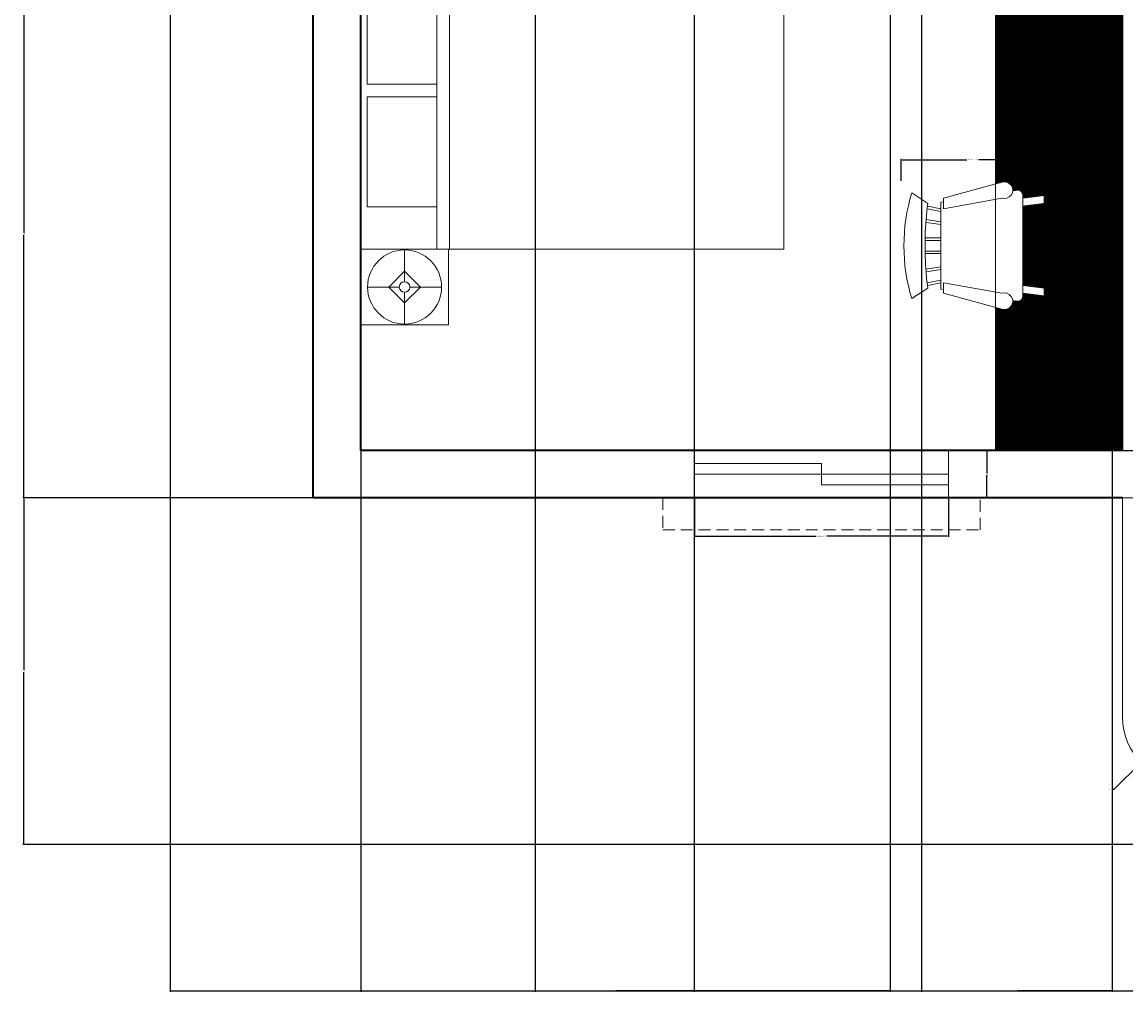
# Model space of a CAD drawing. Units: inches. Extents: x 6662 to 7211, y 5077 to 5683.
# Tile 1 of 9: x 6662 to 6870, y 5077 to 5260. Entities that reach past the tile are written whole.
import ezdxf

# ---------------------------------------------------------------- set-up
doc = ezdxf.new("R2010")
doc.units = ezdxf.units.IN
doc.header["$LTSCALE"] = 3
doc.header["$MEASUREMENT"] = 0
doc.linetypes.add('HIDDEN', pattern=[0.375, 0.25, -0.125])
for name, color, linetype, lineweight in [('A-ANNO-DIMS', 2, 'Continuous', 18), ('A-FLOR-CASE', 8, 'Continuous', 20), ('A-FLOR-CASE-PATT', 241, 'Continuous', 13), ('A-FLOR-HRAL', 7, 'Continuous', 18), ('A-FURN', 8, 'Continuous', 18), ('A-GLAZ', 4, 'Continuous', 18), ('A-GLAZ-OVHD', 4, 'HIDDEN', 13), ('A-WALL', 7, 'Continuous', 35)]:
    doc.layers.add(name, color=color, linetype=linetype, lineweight=lineweight)
doc.styles.get("Standard").update_dxf_attribs({"font": 'arial.ttf'})
doc.dimstyles.get("Standard").update_dxf_attribs({"dimtxt": 0.18, "dimasz": 0.18, "dimexe": 0.18, "dimexo": 0.0625, "dimgap": 0.09, "dimtad": 0, "dimtih": 1, "dimtoh": 1, "dimdec": 4, "dimzin": 0, "dimdsep": 46, "dimtxsty": 'Standard', "dimcen": 0.09, "dimadec": 0, "dimazin": 0, "dimtfac": 1, "dimtdec": 4, "dimtofl": 0, "dimtmove": 0, "dimatfit": 3, "dimfxl": 1, "dimtolj": 1, "dimtzin": 0, "dimarcsym": 0})

# ---------------------------------------------------------------- blocks, each defined once
blk = doc.blocks.new('Chair - Rocking')
for p, q in [((-8, -4.5), (-10, -1.5)), ((8, -4.5), (10, -1.5)), ((-4, -7), (-4.40532, -4.16272)), ((-1.5, -4.05012), (-1.5, -7)), ((-1, -7), (-1, -4.05012)), ((1, -7), (1, -4.04655)), ((1.5, -4.05012), (1.5, -7)), ((-7.5, -4.5), (-7, -7)), ((-6.5, -7), (-7.02225, -4.43)), ((-4.5, -7), (-4.96674, -4.19951)), ((4, -7), (4.40187, -4.18694)), ((4.5, -7), (4.96761, -4.19437)), ((6.5, -7), (7, -4.4057)), ((7.5, -4.5), (7, -7)), ((-9, -7.5), (-12, -18.49999)), ((-7, -7.5), (-9, -7.5)), ((-9, -18.49999), (-7, -7.5)), ((-8.23428, -6.99939), (-8.3093, -7.47958)), ((-8.23041, -7), (8.23915, -7)), ((7, -7.5), (9, -7.5)), ((9, -18.49999), (7, -7.5)), ((8.31071, -7.48854), (8.23449, -7.00073)), ((9, -7.5), (12, -18.49999)), ((-10.36644, -20.64523), (-10.5, -21.49999)), ((10.5, -21.49999), (10.3575, -20.58798)), ((-9, -22.49999), (-9.5, -26.49999)), ((0, -22.49999), (-9.5, -22.49999)), ((-8, -26.49999), (-7.5, -22.49999)), ((0, -22.49999), (9.5, -22.49999)), ((8, -26.49999), (7.5, -22.49999)), ((9, -22.49999), (9.5, -26.49999)), ((-9.5, -26.49999), (-8, -26.49999)), ((9.5, -26.49999), (8, -26.49999))]:
    blk.add_line(p, q)
for centre, radius, start, end in [((0, -34.08333), 34.08333, 72.93847, 107.0615), ((0, -68.25004), 64.25, 93.92211, 97.15267), ((0, -68.25004), 64.25, 82.84733, 93.92211), ((-10.5, -18.99999), 1.58114, 161.5651, 18.43495), ((10.5, -18.99999), 1.58114, 161.5651, 18.43495), ((-9.5, -21.49999), 1, 180, 270), ((9.5, -21.49999), 1, 270, 0)]:
    blk.add_arc(centre, radius, start, end)
blk = doc.blocks.new('Bed - Queen')
for p, q in [((0, -80.00003), (0, 0)), ((0, 0), (59.99999, 0)), ((59.99999, 0), (59.99999, -80.00003)), ((7.99999, -1.2), (28.79998, -1.2)), ((7.99999, -14.4), (7.99999, -1.2)), ((28.79998, -1.2), (28.79998, -14.4)), ((31.19999, -1.2), (51.99999, -1.2)), ((31.19999, -14.4), (31.19999, -1.2)), ((51.99999, -1.2), (51.99999, -16.4)), ((0, -14.4), (44.8, -14.4)), ((59.99999, -29.6), (44.8, -14.4)), ((44.8, -14.4), (44.8, -29.6)), ((51.99999, -16.4), (46.79936, -16.4)), ((44.8, -16.8), (0, -16.8)), ((44.8, -29.6), (59.99999, -29.6)), ((59.99999, -80.00003), (0, -80.00003))]:
    blk.add_line(p, q)
blk = doc.blocks.new('Lamp - Table')
for p, q in [((0, 7), (0, 1)), ((0, 3), (-3, 0)), ((3, 0), (0, 3)), ((-1, 0), (-7, 0)), ((-3, 0), (0, -3)), ((0, -3), (3, 0)), ((1, 0), (7, 0)), ((0, -1), (0, -7))]:
    blk.add_line(p, q)
for radius in [7, 1]:
    blk.add_circle((0, 0), radius)
blk = doc.blocks.new('WIN-SLIDER-48IN')
for p, q in [((0, 0), (0, 9)), ((48, 0), (48, 9)), ((0, 6.5), (24, 6.5)), ((24, 2.5), (24, 6.5)), ((0, 4.5), (48, 4.5)), ((24, 2.5), (48, 2.5))]:
    blk.add_line(p, q)
blk = doc.blocks.new('WIN-HOOD-48IN')
at = {"ltscale": 3}
for p, q in [((0, 0), (0, 6)), ((0, 6), (54, 6)), ((54, 6), (60, 6)), ((60, 6), (60, 0)), ((6, 0), (0, 0))]:
    blk.add_line(p, q, dxfattribs=at)
blk = doc.blocks.new('BEDSIDE-TABLE')
blk.add_lwpolyline([(0, 14.35), (16.56, 14.35), (16.56, 0), (0, 0)], close=True)
blk = doc.blocks.new('*D20')
at = {"layer": 'A-ANNO-DIMS', "color": 0, "lineweight": -2, "ltscale": 3, "transparency": 16777216}
for p, q in [((6828.02, 5230.06), (6828.02, 5234.23)), ((6828.2, 5234.05), (6840.42, 5234.05)), ((6854.84, 5234.05), (6842.61, 5234.05)), ((6855.02, 5230.06), (6855.02, 5234.23))]:
    blk.add_line(p, q, dxfattribs=at)
at = {"layer": 'A-ANNO-DIMS', "color": 0, "ltscale": 3, "transparency": 16777216}
for points in [[(6828.2, 5234.08), (6828.2, 5234.02), (6828.02, 5234.05)], [(6854.84, 5234.08), (6854.84, 5234.02), (6855.02, 5234.05)]]:
    blk.add_solid(points, dxfattribs=at)
at = {"layer": 'Defpoints', "color": 0, "ltscale": 3, "transparency": 16777216}
for p in [(6828.02, 5234.05), (6828.02, 5230), (6855.02, 5230)]:
    blk.add_point(p, dxfattribs=at)
at = {"layer": 'A-ANNO-DIMS', "color": 0, "ltscale": 3, "transparency": 16777216, "insert": (6841.52, 5234.05), "char_height": 0.18, "attachment_point": 5}
blk.add_mtext('\\A1;ROCKER 27 TYP.', dxfattribs=at)
blk = doc.blocks.new('*D21')
at = {"layer": 'A-ANNO-DIMS', "color": 0, "lineweight": -2, "ltscale": 3, "transparency": 16777216}
for p, q in [((6855.08, 5230), (6859.25, 5230)), ((6859.07, 5229.82), (6859.07, 5217.96)), ((6859.07, 5205.74), (6859.07, 5217.6)), ((6855.08, 5205.56), (6859.25, 5205.56))]:
    blk.add_line(p, q, dxfattribs=at)
at = {"layer": 'A-ANNO-DIMS', "color": 0, "ltscale": 3, "transparency": 16777216}
for points in [[(6859.04, 5229.82), (6859.1, 5229.82), (6859.07, 5230)], [(6859.04, 5205.74), (6859.1, 5205.74), (6859.07, 5205.56)]]:
    blk.add_solid(points, dxfattribs=at)
at = {"layer": 'Defpoints', "color": 0, "ltscale": 3, "transparency": 16777216}
for p in [(6855.02, 5230), (6859.07, 5230), (6855.02, 5205.56)]:
    blk.add_point(p, dxfattribs=at)
at = {"layer": 'A-ANNO-DIMS', "color": 0, "ltscale": 3, "transparency": 16777216, "insert": (6859.07, 5217.78), "char_height": 0.18, "attachment_point": 5}
blk.add_mtext('\\A1;24 TYP.', dxfattribs=at)
blk = doc.blocks.new('*D24')
at = {"layer": 'A-ANNO-DIMS', "color": 0, "lineweight": -2, "ltscale": 3, "transparency": 16777216}
for p, q in [((6788.97, 5170.04), (6788.97, 5162.72)), ((6836.97, 5170.04), (6836.97, 5162.72)), ((6789.15, 5162.9), (6811.95, 5162.9)), ((6836.79, 5162.9), (6813.98, 5162.9))]:
    blk.add_line(p, q, dxfattribs=at)
at = {"layer": 'A-ANNO-DIMS', "color": 0, "ltscale": 3, "transparency": 16777216}
for points in [[(6789.15, 5162.93), (6789.15, 5162.87), (6788.97, 5162.9)], [(6836.79, 5162.93), (6836.79, 5162.87), (6836.97, 5162.9)]]:
    blk.add_solid(points, dxfattribs=at)
at = {"layer": 'Defpoints', "color": 0, "ltscale": 3, "transparency": 16777216}
for p in [(6788.97, 5170.1), (6836.97, 5170.1), (6788.97, 5162.9)]:
    blk.add_point(p, dxfattribs=at)
at = {"layer": 'A-ANNO-DIMS', "color": 0, "ltscale": 3, "transparency": 16777216, "insert": (6812.97, 5162.9), "char_height": 0.18, "attachment_point": 5}
blk.add_mtext('\\A1;SLIDER 48 TYP.', dxfattribs=at)
blk = doc.blocks.new('*D25')
at = {"layer": 'A-ANNO-DIMS', "color": 0, "lineweight": -2, "ltscale": 3, "transparency": 16777216}
for p, q in [((6837.03, 5179.1), (6844.35, 5179.1)), ((6844.17, 5178.92), (6844.17, 5174.78)), ((6844.17, 5170.28), (6844.17, 5174.42)), ((6837.03, 5170.1), (6844.35, 5170.1))]:
    blk.add_line(p, q, dxfattribs=at)
at = {"layer": 'A-ANNO-DIMS', "color": 0, "ltscale": 3, "transparency": 16777216}
for points in [[(6844.14, 5178.92), (6844.2, 5178.92), (6844.17, 5179.1)], [(6844.14, 5170.28), (6844.2, 5170.28), (6844.17, 5170.1)]]:
    blk.add_solid(points, dxfattribs=at)
at = {"layer": 'Defpoints', "color": 0, "ltscale": 3, "transparency": 16777216}
for p in [(6836.97, 5179.1), (6836.97, 5170.1), (6844.17, 5170.1)]:
    blk.add_point(p, dxfattribs=at)
at = {"layer": 'A-ANNO-DIMS', "color": 0, "ltscale": 3, "transparency": 16777216, "insert": (6844.17, 5174.6), "char_height": 0.18, "attachment_point": 5}
blk.add_mtext('\\A1;9 TYP.', dxfattribs=at)
blk = doc.blocks.new('*D40')
at = {"layer": 'A-ANNO-DIMS', "color": 0, "lineweight": -2, "ltscale": 3, "transparency": 16777216}
for p, q in [((7182.86, 5326.04), (7182.86, 5076.72)), ((6689.86, 5323.04), (6689.86, 5076.72)), ((6690.04, 5076.9), (6936.07, 5076.9)), ((7182.68, 5076.9), (6936.65, 5076.9))]:
    blk.add_line(p, q, dxfattribs=at)
at = {"layer": 'A-ANNO-DIMS', "color": 0, "ltscale": 3, "transparency": 16777216}
for points in [[(6690.04, 5076.93), (6690.04, 5076.87), (6689.86, 5076.9)], [(7182.68, 5076.93), (7182.68, 5076.87), (7182.86, 5076.9)]]:
    blk.add_solid(points, dxfattribs=at)
at = {"layer": 'Defpoints', "color": 0, "ltscale": 3, "transparency": 16777216}
for p in [(7182.86, 5326.1), (6689.86, 5323.1), (7182.86, 5076.9)]:
    blk.add_point(p, dxfattribs=at)
at = {"layer": 'A-ANNO-DIMS', "color": 0, "ltscale": 3, "transparency": 16777216, "insert": (6936.36, 5076.9), "char_height": 0.18, "attachment_point": 5}
blk.add_mtext('\\A1;493', dxfattribs=at)
blk = doc.blocks.new('*D59')
at = {"layer": 'A-ANNO-DIMS', "color": 0, "lineweight": -2, "ltscale": 3, "transparency": 16777216}
for p, q in [((6716.8, 5269.94), (6661.98, 5269.94)), ((6662.16, 5269.76), (6662.16, 5220.2)), ((6662.16, 5170.28), (6662.16, 5219.84)), ((6716.8, 5170.1), (6661.98, 5170.1))]:
    blk.add_line(p, q, dxfattribs=at)
at = {"layer": 'A-ANNO-DIMS', "color": 0, "ltscale": 3, "transparency": 16777216}
for points in [[(6662.13, 5269.76), (6662.19, 5269.76), (6662.16, 5269.94)], [(6662.13, 5170.28), (6662.19, 5170.28), (6662.16, 5170.1)]]:
    blk.add_solid(points, dxfattribs=at)
at = {"layer": 'Defpoints', "color": 0, "ltscale": 3, "transparency": 16777216}
for p in [(6716.86, 5269.94), (6662.16, 5170.1), (6716.86, 5170.1)]:
    blk.add_point(p, dxfattribs=at)
at = {"layer": 'A-ANNO-DIMS', "color": 0, "ltscale": 3, "transparency": 16777216, "insert": (6662.16, 5220.02), "char_height": 0.18, "attachment_point": 5}
blk.add_mtext('\\A1;99.84', dxfattribs=at)
blk = doc.blocks.new('*D60')
at = {"layer": 'A-ANNO-DIMS', "color": 0, "lineweight": -2, "ltscale": 3, "transparency": 16777216}
for p, q in [((6716.8, 5170.1), (6661.98, 5170.1)), ((6662.16, 5169.92), (6662.16, 5137.53)), ((6662.16, 5104.78), (6662.16, 5137.17)), ((7001.8, 5104.6), (6661.98, 5104.6))]:
    blk.add_line(p, q, dxfattribs=at)
at = {"layer": 'A-ANNO-DIMS', "color": 0, "ltscale": 3, "transparency": 16777216}
for points in [[(6662.13, 5169.92), (6662.19, 5169.92), (6662.16, 5170.1)], [(6662.13, 5104.78), (6662.19, 5104.78), (6662.16, 5104.6)]]:
    blk.add_solid(points, dxfattribs=at)
at = {"layer": 'Defpoints', "color": 0, "ltscale": 3, "transparency": 16777216}
for p in [(6716.86, 5170.1), (6662.16, 5104.6), (7001.86, 5104.6)]:
    blk.add_point(p, dxfattribs=at)
at = {"layer": 'A-ANNO-DIMS', "color": 0, "ltscale": 3, "transparency": 16777216, "insert": (6662.16, 5137.35), "char_height": 0.18, "attachment_point": 5}
blk.add_mtext('\\A1;65.5', dxfattribs=at)
blk = doc.blocks.new('*D62')
at = {"layer": 'A-ANNO-DIMS', "color": 0, "lineweight": -2, "ltscale": 3, "transparency": 16777216}
for p, q in [((6758.86, 5388.04), (6758.86, 5076.72)), ((6788.86, 5388.04), (6788.86, 5076.72)), ((6759.04, 5076.9), (6773.64, 5076.9)), ((6788.68, 5076.9), (6774.08, 5076.9))]:
    blk.add_line(p, q, dxfattribs=at)
at = {"layer": 'A-ANNO-DIMS', "color": 0, "ltscale": 3, "transparency": 16777216}
for points in [[(6759.04, 5076.93), (6759.04, 5076.87), (6758.86, 5076.9)], [(6788.68, 5076.93), (6788.68, 5076.87), (6788.86, 5076.9)]]:
    blk.add_solid(points, dxfattribs=at)
at = {"layer": 'Defpoints', "color": 0, "ltscale": 3, "transparency": 16777216}
for p in [(6758.86, 5388.1), (6788.86, 5388.1), (6788.86, 5076.9)]:
    blk.add_point(p, dxfattribs=at)
at = {"layer": 'A-ANNO-DIMS', "color": 0, "ltscale": 3, "transparency": 16777216, "insert": (6773.86, 5076.9), "char_height": 0.18, "attachment_point": 5}
blk.add_mtext('\\A1;30', dxfattribs=at)
blk = doc.blocks.new('*D65')
at = {"layer": 'A-ANNO-DIMS', "color": 0, "lineweight": -2, "ltscale": 3, "transparency": 16777216}
for p, q in [((6831.86, 5464.54), (6831.86, 5076.72)), ((6867.86, 5464.54), (6867.86, 5076.72)), ((6832.04, 5076.9), (6849.64, 5076.9)), ((6867.68, 5076.9), (6850.08, 5076.9))]:
    blk.add_line(p, q, dxfattribs=at)
at = {"layer": 'A-ANNO-DIMS', "color": 0, "ltscale": 3, "transparency": 16777216}
for points in [[(6832.04, 5076.93), (6832.04, 5076.87), (6831.86, 5076.9)], [(6867.68, 5076.93), (6867.68, 5076.87), (6867.86, 5076.9)]]:
    blk.add_solid(points, dxfattribs=at)
at = {"layer": 'Defpoints', "color": 0, "ltscale": 3, "transparency": 16777216}
for p in [(6831.86, 5464.6), (6867.86, 5464.6), (6867.86, 5076.9)]:
    blk.add_point(p, dxfattribs=at)
at = {"layer": 'A-ANNO-DIMS', "color": 0, "ltscale": 3, "transparency": 16777216, "insert": (6849.86, 5076.9), "char_height": 0.18, "attachment_point": 5}
blk.add_mtext('\\A1;36', dxfattribs=at)
blk = doc.blocks.new('*D73')
at = {"layer": 'A-ANNO-DIMS', "color": 0, "lineweight": -2, "ltscale": 3, "transparency": 16777216}
for p, q in [((6725.86, 5179.16), (6725.86, 5682.9)), ((6726.04, 5682.72), (6757.03, 5682.72)), ((6788.79, 5682.72), (6757.79, 5682.72)), ((6788.97, 5179.16), (6788.97, 5682.9))]:
    blk.add_line(p, q, dxfattribs=at)
at = {"layer": 'A-ANNO-DIMS', "color": 0, "ltscale": 3, "transparency": 16777216}
for points in [[(6726.04, 5682.75), (6726.04, 5682.69), (6725.86, 5682.72)], [(6788.79, 5682.75), (6788.79, 5682.69), (6788.97, 5682.72)]]:
    blk.add_solid(points, dxfattribs=at)
at = {"layer": 'Defpoints', "color": 0, "ltscale": 3, "transparency": 16777216}
for p in [(6788.97, 5682.72), (6725.86, 5179.1), (6788.97, 5179.1)]:
    blk.add_point(p, dxfattribs=at)
at = {"layer": 'A-ANNO-DIMS', "color": 0, "ltscale": 3, "transparency": 16777216, "insert": (6757.41, 5682.72), "char_height": 0.18, "attachment_point": 5}
blk.add_mtext('\\A1;63.11', dxfattribs=at)
blk = doc.blocks.new('*D79')
at = {"layer": 'A-ANNO-DIMS', "color": 0, "lineweight": -2, "ltscale": 3, "transparency": 16777216}
for p, q in [((6725.86, 5473.54), (6725.86, 5076.72)), ((6825.9, 5473.54), (6825.9, 5076.72)), ((6726.04, 5076.9), (6775.42, 5076.9)), ((6825.72, 5076.9), (6776.33, 5076.9))]:
    blk.add_line(p, q, dxfattribs=at)
at = {"layer": 'A-ANNO-DIMS', "color": 0, "ltscale": 3, "transparency": 16777216}
for points in [[(6726.04, 5076.93), (6726.04, 5076.87), (6725.86, 5076.9)], [(6825.72, 5076.93), (6825.72, 5076.87), (6825.9, 5076.9)]]:
    blk.add_solid(points, dxfattribs=at)
at = {"layer": 'Defpoints', "color": 0, "ltscale": 3, "transparency": 16777216}
for p in [(6725.86, 5473.6), (6825.9, 5473.6), (6825.9, 5076.9)]:
    blk.add_point(p, dxfattribs=at)
at = {"layer": 'A-ANNO-DIMS', "color": 0, "ltscale": 3, "transparency": 16777216, "insert": (6775.88, 5076.9), "char_height": 0.18, "attachment_point": 5}
blk.add_mtext('\\A1;100.04', dxfattribs=at)
blk = doc.blocks.new('*D83')
at = {"layer": 'A-ANNO-DIMS', "color": 0, "lineweight": -2, "ltscale": 3, "transparency": 16777216}
for p, q in [((6845.92, 5283.8), (7210.74, 5283.8)), ((7210.56, 5283.62), (7210.56, 5231.63)), ((7210.56, 5179.28), (7210.56, 5231.27)), ((6845.92, 5179.1), (7210.74, 5179.1))]:
    blk.add_line(p, q, dxfattribs=at)
at = {"layer": 'A-ANNO-DIMS', "color": 0, "ltscale": 3, "transparency": 16777216}
for points in [[(7210.53, 5283.62), (7210.59, 5283.62), (7210.56, 5283.8)], [(7210.53, 5179.28), (7210.59, 5179.28), (7210.56, 5179.1)]]:
    blk.add_solid(points, dxfattribs=at)
at = {"layer": 'Defpoints', "color": 0, "ltscale": 3, "transparency": 16777216}
for p in [(6845.86, 5283.8), (7210.56, 5283.8), (6845.86, 5179.1)]:
    blk.add_point(p, dxfattribs=at)
at = {"layer": 'A-ANNO-DIMS', "color": 0, "ltscale": 3, "transparency": 16777216, "insert": (7210.56, 5231.45), "char_height": 0.18, "attachment_point": 5}
blk.add_mtext('\\A1;104.7', dxfattribs=at)
blk = doc.blocks.new('*D87')
at = {"layer": 'A-ANNO-DIMS', "color": 0, "lineweight": -2, "ltscale": 3, "transparency": 16777216}
for p, q in [((6881.77, 5128.6), (6881.95, 5128.6)), ((6881.86, 5128.51), (6881.86, 5128.69)), ((6868.28, 5115.02), (6873.25, 5119.99)), ((6868.1, 5115.02), (6868.28, 5115.02))]:
    blk.add_line(p, q, dxfattribs=at)
at = {"layer": 'A-ANNO-DIMS', "color": 0, "ltscale": 3, "transparency": 16777216}
blk.add_solid([(6873.22, 5120.01), (6873.27, 5119.96), (6873.37, 5120.11)], dxfattribs=at)
at = {"layer": 'Defpoints', "color": 0, "ltscale": 3, "transparency": 16777216}
for p in [(6881.86, 5128.6), (6873.37, 5120.11)]:
    blk.add_point(p, dxfattribs=at)
at = {"layer": 'A-ANNO-DIMS', "color": 0, "ltscale": 3, "transparency": 16777216, "insert": (6867.6, 5115.02), "char_height": 0.18, "attachment_point": 5}
blk.add_mtext('\\A1;2X R12', dxfattribs=at)

msp = doc.modelspace()

# ---------------------------------------------------------------- hatches: boundary and pattern name
at = {"layer": 'A-FLOR-CASE-PATT'}
h = msp.add_hatch(dxfattribs=at)
h.set_pattern_fill('ANSI31', color=256)
h.paths.add_polyline_path([(6869.8579, 5283.7981), (6845.8579, 5283.7981), (6845.8579, 5229.4653), (6847.018, 5229.7817, -0.54116316), (6849.0925, 5228.1371), (6849.7129, 5228.234, -0.50821327), (6851.018, 5227.2817), (6851.018, 5226.7817), (6855.018, 5227.2817), (6855.018, 5225.7817), (6851.018, 5225.2817), (6851.018, 5217.7817), (6851.018, 5210.2817), (6855.018, 5209.7817), (6855.018, 5208.2817), (6851.018, 5208.7817), (6851.018, 5208.2817, -0.41421356), (6850.018, 5207.2817), (6849.0925, 5207.4263, -0.50580924), (6847.1872, 5205.7355), (6845.8579, 5206.0981), (6845.8579, 5179.0979), (6869.8579, 5179.0979)])
h.paths.add_polyline_path([(7167.8579, 5497.5979), (7143.8579, 5497.5979), (7078.3579, 5497.5979), (7078.3579, 5473.5979), (7163.8579, 5473.5979), (7167.8579, 5473.5979)])
h.paths.add_polyline_path([(6825.9016, 5497.5979), (6725.8579, 5497.5979), (6725.8579, 5473.5979), (6825.9016, 5473.5979)])
h.paths.add_polyline_path([(6796.6359, 5485.2095), (6797.1359, 5489.2095), (6806.1359, 5489.2095), (6815.1359, 5489.2095), (6815.6359, 5485.2095), (6814.1359, 5485.2095), (6813.6359, 5489.2095), (6806.1359, 5489.2095), (6798.6359, 5489.2095), (6798.1359, 5485.2095)], flags=16)

# ---------------------------------------------------------------- linework, layer by layer
at = {"layer": 'A-FLOR-CASE'}
msp.add_line((6845.8579, 5179.0979), (6845.8579, 5283.7981), dxfattribs=at)
at = {"layer": 'A-FLOR-HRAL'}
for p, q in [((6869.8579, 5128.5979), (6869.8579, 5170.0979)), ((6869.8579, 5170.0979), (6878.8579, 5170.0979))]:
    msp.add_line(p, q, dxfattribs=at)
msp.add_arc((6881.8579, 5128.5979), 12, 180, 270, dxfattribs=at)
at = {"layer": 'A-WALL'}
for p, q in [((6716.8579, 5170.0979), (6716.8579, 5626.5979)), ((6725.8579, 5179.0979), (6725.8579, 5323.0979)), ((6869.8579, 5179.0979), (6869.8579, 5323.0979)), ((6869.8579, 5179.0979), (6725.8579, 5179.0979)), ((6869.8579, 5170.0979), (6716.8579, 5170.0979))]:
    msp.add_line(p, q, dxfattribs=at)

# ---------------------------------------------------------------- block references
at = {"layer": 'A-FURN', "rotation": 90}
for name, p in [('Bed - Queen', (6725.8579, 5217.1528)), ('Chair - Rocking', (6828.518, 5217.7817))]:
    msp.add_blockref(name, p, dxfattribs=at)
at = {"layer": 'A-FURN'}
for name, p in [('BEDSIDE-TABLE', (6725.858, 5202.8)), ('Lamp - Table', (6734.1467, 5209.9762))]:
    msp.add_blockref(name, p, dxfattribs=at)
at = {"layer": 'A-GLAZ', "rotation": 180}
msp.add_blockref('WIN-SLIDER-48IN', (6836.9656, 5179.0979), dxfattribs=at)
at = {"layer": 'A-GLAZ-OVHD', "extrusion": (0, 0, -1), "zscale": -1, "rotation": 180}
msp.add_blockref('WIN-HOOD-48IN', (-6782.9658, 5170.0979), dxfattribs=at)

# ---------------------------------------------------------------- dimensions: what is measured, and where the dimension line sits
at = {"layer": 'A-ANNO-DIMS', "ltscale": 3}
for base, p1, p2, override, picture, middle in [((6788.9657, 5682.7209), (6725.8579, 5179.0979), (6788.9657, 5179.0979), {"dimdec": 2, "dimlfac": 1, "dimrnd": 0, "dimzin": 0, "dimdsep": 46, "dimlunit": 2}, '*D73', (6757.4118, 5682.7209)), ((6825.9016, 5076.8979), (6725.8579, 5473.5979), (6825.9016, 5473.5979), {"dimdec": 2, "dimlfac": 1, "dimrnd": 0, "dimzin": 0, "dimdsep": 46, "dimlunit": 2}, '*D79', (6775.8797, 5076.8979)), ((6867.8579, 5076.8979), (6831.8579, 5464.5979), (6867.8579, 5464.5979), {"dimdec": 0, "dimlfac": 1, "dimrnd": 0, "dimzin": 0, "dimdsep": 46, "dimlunit": 2}, '*D65', (6849.8579, 5076.8979)), ((6788.8579, 5076.8979), (6758.8579, 5388.0979), (6788.8579, 5388.0979), {"dimdec": 0, "dimlfac": 1, "dimrnd": 0, "dimzin": 0, "dimdsep": 46, "dimlunit": 2}, '*D62', (6773.8579, 5076.8979)), ((7182.8579, 5076.8979), (6689.8579, 5323.0979), (7182.8579, 5326.0979), {"dimdec": 0, "dimlfac": 1, "dimrnd": 0, "dimzin": 0, "dimdsep": 46, "dimlunit": 2}, '*D40', (6936.3579, 5076.8979))]:
    dim = msp.add_linear_dim(base=base, p1=p1, p2=p2, dimstyle='Standard', override=override, dxfattribs=at)
    dim.commit()
    dim.dimension.update_dxf_attribs({"geometry": picture, "text_midpoint": middle})
for base, p1, p2, override, picture, middle in [((7210.5579, 5283.7981), (6845.8579, 5179.0979), (6845.8579, 5283.7981), {"dimdec": 1, "dimlfac": 1, "dimrnd": 0, "dimzin": 0, "dimdsep": 46, "dimlunit": 2}, '*D83', (7210.5579, 5231.448)), ((6662.1579, 5170.0979), (6716.8579, 5269.94), (6716.8579, 5170.0979), {"dimdec": 2, "dimlfac": 1, "dimrnd": 0, "dimzin": 0, "dimdsep": 46, "dimlunit": 2}, '*D59', (6662.1579, 5220.019)), ((6662.1579, 5104.5979), (6716.8579, 5170.0979), (7001.8579, 5104.5979), {"dimdec": 1, "dimlfac": 1, "dimrnd": 0, "dimzin": 0, "dimdsep": 46, "dimlunit": 2}, '*D60', (6662.1579, 5137.3479))]:
    dim = msp.add_linear_dim(base=base, p1=p1, p2=p2, angle=90, dimstyle='Standard', override=override, dxfattribs=at)
    dim.commit()
    dim.dimension.update_dxf_attribs({"geometry": picture, "text_midpoint": middle})
for base, p1, p2, angle, text, picture, middle in [((6828.018, 5234.0492), (6855.018, 5229.9993), (6828.018, 5229.9993), 180, 'ROCKER <> TYP.', '*D20', (6841.518, 5234.0492)), ((6859.068, 5229.9993), (6855.018, 5205.5642), (6855.018, 5229.9993), 90, '<> TYP.', '*D21', (6859.068, 5217.7817)), ((6844.1657, 5170.0979), (6836.9657, 5179.0979), (6836.9657, 5170.0979), 270, '<> TYP.', '*D25', (6844.1657, 5174.5979)), ((6788.9657, 5162.8979), (6836.9657, 5170.0979), (6788.9657, 5170.0979), 180, 'SLIDER <> TYP.', '*D24', (6812.9657, 5162.8979))]:
    dim = msp.add_linear_dim(base=base, p1=p1, p2=p2, angle=angle, text=text, dimstyle='Standard', override={"dimdec": 0, "dimlfac": 1, "dimrnd": 0, "dimzin": 0, "dimdsep": 46, "dimlunit": 2}, dxfattribs=at)
    dim.commit()
    dim.dimension.update_dxf_attribs({"geometry": picture, "text_midpoint": middle})
dim = msp.add_radius_dim(center=(6881.8579, 5128.5979), mpoint=(6873.3726, 5120.1126), text='2X <>', dimstyle='Standard', override={"dimdec": 0, "dimlfac": 1, "dimrnd": 0, "dimzin": 0, "dimdsep": 46, "dimlunit": 2}, dxfattribs=at)
dim.commit()
dim.dimension.update_dxf_attribs({"geometry": '*D87', "text_midpoint": (6867.6024, 5115.0214), "dimtype": 164})

doc.saveas('drawing.dxf')
